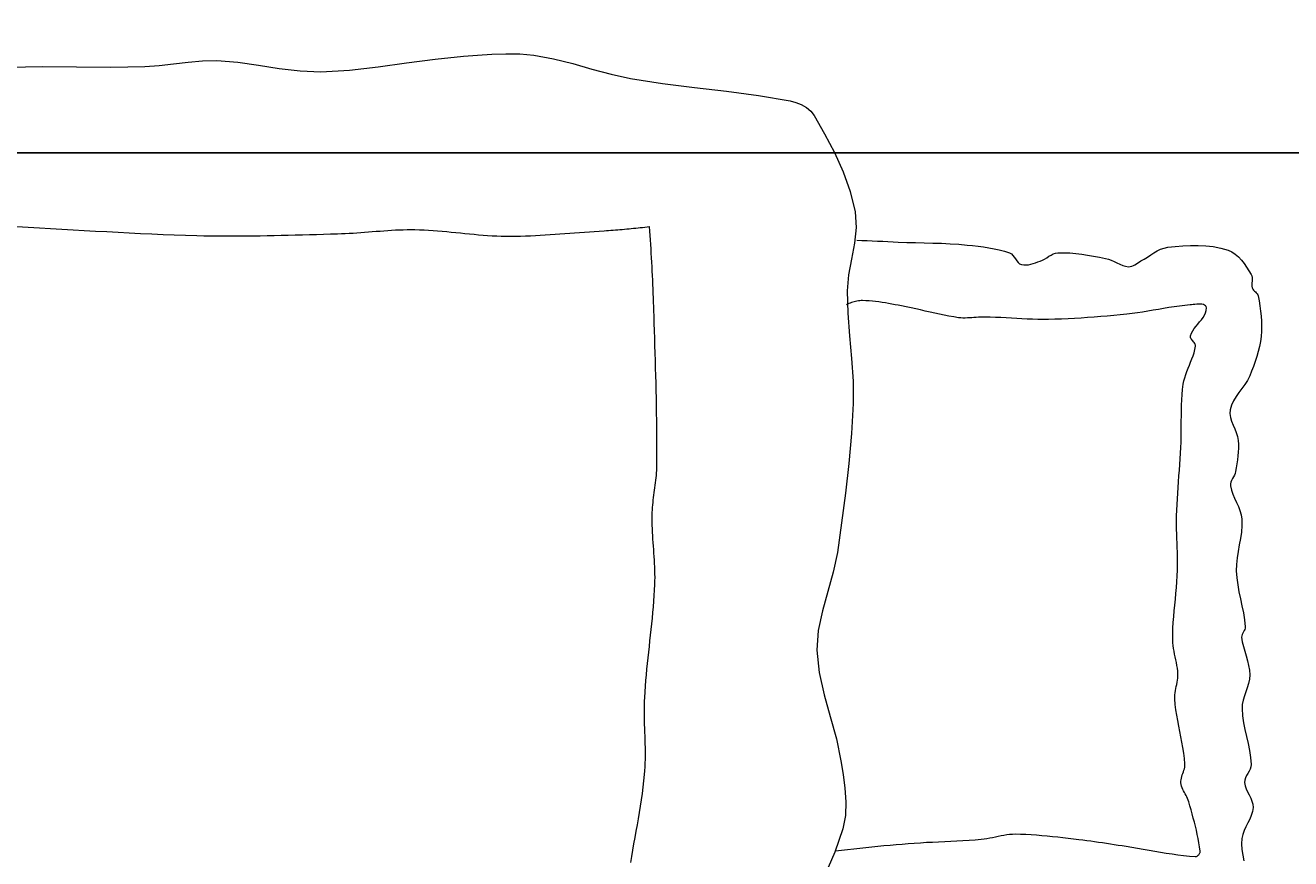
# Model space of a CAD drawing. Units: inches. Extents: x -15 to 423, y -713 to 71.
# Tile 15 of 24: x 308 to 364, y -308 to -270. Entities that reach past the tile are written whole.
import ezdxf

# ---------------------------------------------------------------- set-up
doc = ezdxf.new("R2010")
doc.units = ezdxf.units.IN
doc.header["$MEASUREMENT"] = 0
doc.layers.add('A-ANNO-DIMS', color=2, linetype='Continuous', lineweight=18)
doc.layers.add('A-FURN', color=9, linetype='Continuous', lineweight=13)
doc.styles.get("Standard").update_dxf_attribs({"font": 'arial.ttf'})
doc.dimstyles.get("Standard").update_dxf_attribs({"dimtxt": 0.18, "dimasz": 0.18, "dimexe": 0.18, "dimexo": 0.0625, "dimgap": 0.09, "dimtad": 0, "dimtih": 1, "dimtoh": 1, "dimdec": 0, "dimzin": 0, "dimdsep": 46, "dimlunit": 3, "dimtxsty": 'Standard', "dimcen": 0.09, "dimadec": 0, "dimazin": 0, "dimtfac": 1, "dimtdec": 0, "dimtofl": 0, "dimtmove": 0, "dimatfit": 3, "dimfxl": 1, "dimtolj": 1, "dimtzin": 0, "dimarcsym": 0})

# ---------------------------------------------------------------- blocks, each defined once
blk = doc.blocks.new('BED-DOUBLE')
for p, q in [((51.556, 70.189), (52.201, 70.268)), ((52.201, 70.268), (52.847, 70.326)), ((52.847, 70.326), (53.495, 70.339)), ((53.495, 70.339), (54.428, 70.266)), ((54.428, 70.266), (55.357, 70.134)), ((61.983, 70.229), (63.259, 70.403)), ((63.259, 70.403), (64.539, 70.536)), ((64.539, 70.536), (65.168, 70.585)), ((65.168, 70.585), (65.8, 70.625)), ((65.8, 70.625), (66.431, 70.645)), ((66.431, 70.645), (67.061, 70.633)), ((67.061, 70.633), (67.688, 70.576)), ((67.688, 70.576), (68.563, 70.418)), ((68.563, 70.418), (69.426, 70.201)), ((44.16, 70.042), (45.684, 70.067)), ((45.684, 70.067), (47.211, 70.055)), ((47.211, 70.055), (48.737, 70.043)), ((48.737, 70.043), (50.262, 70.068)), ((50.262, 70.068), (50.909, 70.114)), ((50.909, 70.114), (51.556, 70.189)), ((55.357, 70.134), (56.285, 69.988)), ((56.285, 69.988), (57.214, 69.874)), ((57.214, 69.874), (58.147, 69.837)), ((58.147, 69.837), (59.429, 69.908)), ((59.429, 69.908), (60.707, 70.052)), ((60.707, 70.052), (61.983, 70.229)), ((69.426, 70.201), (70.285, 69.959)), ((70.285, 69.959), (71.146, 69.727)), ((71.146, 69.727), (72.016, 69.538)), ((72.016, 69.538), (73.443, 69.316)), ((73.443, 69.316), (74.876, 69.137)), ((74.876, 69.137), (76.311, 68.967)), ((76.311, 68.967), (77.741, 68.775)), ((77.741, 68.775), (79.163, 68.528)), ((79.163, 68.528), (79.412, 68.464)), ((79.412, 68.464), (79.657, 68.368)), ((79.657, 68.368), (79.885, 68.24)), ((79.885, 68.24), (80.082, 68.078)), ((80.082, 68.078), (80.236, 67.88)), ((80.236, 67.88), (80.703, 67.06)), ((80.703, 67.06), (81.141, 66.219)), ((81.141, 66.219), (81.529, 65.356)), ((81.529, 65.356), (81.847, 64.47)), ((81.847, 64.47), (82.074, 63.56)), ((82.074, 63.56), (82.122, 62.86)), ((44.535, 62.904), (45.039, 62.877)), ((72.754, 62.888), (72.855, 62.9)), ((72.855, 62.9), (72.869, 62.701)), ((45.039, 62.877), (45.543, 62.849)), ((45.543, 62.849), (46.046, 62.82)), ((46.046, 62.82), (46.55, 62.791)), ((46.55, 62.791), (47.053, 62.762)), ((47.053, 62.762), (47.557, 62.732)), ((47.557, 62.732), (48.06, 62.703)), ((48.06, 62.703), (48.564, 62.675)), ((48.564, 62.675), (49.068, 62.647)), ((49.068, 62.647), (49.571, 62.62)), ((49.571, 62.62), (50.075, 62.595)), ((50.075, 62.595), (50.579, 62.572)), ((50.579, 62.572), (51.083, 62.55)), ((51.083, 62.55), (51.586, 62.53)), ((51.586, 62.53), (52.09, 62.513)), ((52.09, 62.513), (52.595, 62.499)), ((52.595, 62.499), (52.909, 62.492)), ((52.909, 62.492), (53.224, 62.487)), ((53.224, 62.487), (53.539, 62.483)), ((53.539, 62.483), (53.854, 62.481)), ((53.854, 62.481), (54.169, 62.481)), ((54.169, 62.481), (54.484, 62.482)), ((54.484, 62.482), (54.799, 62.484)), ((54.799, 62.484), (55.114, 62.488)), ((55.114, 62.488), (55.429, 62.492)), ((55.429, 62.492), (55.744, 62.497)), ((55.744, 62.497), (56.059, 62.504)), ((56.059, 62.504), (56.374, 62.511)), ((56.374, 62.511), (56.689, 62.518)), ((56.689, 62.518), (57.004, 62.526)), ((57.004, 62.526), (57.319, 62.535)), ((57.319, 62.535), (57.634, 62.543)), ((57.634, 62.543), (57.949, 62.552)), ((57.949, 62.552), (58.264, 62.561)), ((58.264, 62.561), (58.579, 62.57)), ((58.579, 62.57), (58.893, 62.579)), ((58.893, 62.579), (59.067, 62.585)), ((59.067, 62.585), (59.24, 62.592)), ((59.24, 62.592), (59.413, 62.602)), ((59.413, 62.602), (59.587, 62.612)), ((59.587, 62.612), (59.76, 62.624)), ((59.76, 62.624), (59.933, 62.637)), ((59.933, 62.637), (60.106, 62.65)), ((60.106, 62.65), (60.279, 62.663)), ((60.279, 62.663), (60.452, 62.677)), ((60.452, 62.677), (60.625, 62.691)), ((60.625, 62.691), (60.798, 62.704)), ((60.798, 62.704), (60.971, 62.717)), ((60.971, 62.717), (61.145, 62.729)), ((61.145, 62.729), (61.318, 62.739)), ((61.318, 62.739), (61.491, 62.749)), ((61.491, 62.749), (61.664, 62.756)), ((61.664, 62.756), (61.837, 62.762)), ((61.837, 62.762), (62.011, 62.766)), ((62.011, 62.766), (62.184, 62.768)), ((62.184, 62.768), (62.357, 62.767)), ((62.357, 62.767), (62.562, 62.762)), ((62.562, 62.762), (62.766, 62.754)), ((62.766, 62.754), (62.969, 62.743)), ((62.969, 62.743), (63.173, 62.73)), ((63.173, 62.73), (63.377, 62.714)), ((63.377, 62.714), (63.58, 62.696)), ((63.58, 62.696), (63.784, 62.677)), ((63.784, 62.677), (63.988, 62.657)), ((63.988, 62.657), (64.191, 62.637)), ((64.191, 62.637), (64.394, 62.616)), ((64.394, 62.616), (64.598, 62.595)), ((64.598, 62.595), (64.801, 62.574)), ((64.801, 62.574), (65.005, 62.555)), ((65.005, 62.555), (65.208, 62.537)), ((65.208, 62.537), (65.412, 62.52)), ((65.412, 62.52), (65.616, 62.505)), ((65.616, 62.505), (65.819, 62.493)), ((65.819, 62.493), (66.023, 62.483)), ((66.023, 62.483), (66.227, 62.476)), ((66.227, 62.476), (66.432, 62.473)), ((66.432, 62.473), (66.652, 62.473)), ((66.652, 62.473), (66.872, 62.475)), ((66.872, 62.475), (67.092, 62.479)), ((67.092, 62.479), (67.312, 62.486)), ((67.312, 62.486), (67.532, 62.494)), ((67.532, 62.494), (67.752, 62.503)), ((67.752, 62.503), (67.972, 62.514)), ((67.972, 62.514), (68.192, 62.527)), ((68.192, 62.527), (68.412, 62.54)), ((68.412, 62.54), (68.632, 62.555)), ((68.632, 62.555), (68.852, 62.57)), ((68.852, 62.57), (69.072, 62.586)), ((69.072, 62.586), (69.291, 62.602)), ((69.291, 62.602), (69.511, 62.619)), ((69.511, 62.619), (69.731, 62.636)), ((69.731, 62.636), (69.951, 62.652)), ((69.951, 62.652), (70.17, 62.669)), ((70.17, 62.669), (70.39, 62.685)), ((70.39, 62.685), (70.61, 62.701)), ((70.61, 62.701), (70.83, 62.716)), ((70.83, 62.716), (70.931, 62.723)), ((70.931, 62.723), (71.033, 62.73)), ((71.033, 62.73), (71.134, 62.737)), ((71.134, 62.737), (71.236, 62.745)), ((71.236, 62.745), (71.337, 62.753)), ((71.337, 62.753), (71.438, 62.761)), ((71.438, 62.761), (71.54, 62.769)), ((71.54, 62.769), (71.641, 62.778)), ((71.641, 62.778), (71.742, 62.787)), ((71.742, 62.787), (71.844, 62.796)), ((71.844, 62.796), (71.945, 62.805)), ((71.945, 62.805), (72.046, 62.814)), ((72.046, 62.814), (72.147, 62.824)), ((72.147, 62.824), (72.249, 62.834)), ((72.249, 62.834), (72.35, 62.845)), ((72.35, 62.845), (72.451, 62.855)), ((72.451, 62.855), (72.552, 62.866)), ((72.552, 62.866), (72.653, 62.877)), ((72.653, 62.877), (72.754, 62.888)), ((72.869, 62.701), (72.882, 62.501)), ((72.882, 62.501), (72.894, 62.302)), ((82.122, 62.86), (82.046, 62.156)), ((72.894, 62.302), (72.906, 62.103)), ((72.906, 62.103), (72.918, 61.903)), ((72.918, 61.903), (72.929, 61.704)), ((82.046, 62.156), (81.91, 61.449)), ((82.14, 62.295), (82.373, 62.284)), ((82.373, 62.284), (82.606, 62.273)), ((82.606, 62.273), (82.839, 62.263)), ((82.839, 62.263), (83.072, 62.252)), ((83.072, 62.252), (83.305, 62.242)), ((83.305, 62.242), (83.538, 62.231)), ((83.538, 62.231), (83.771, 62.221)), ((83.771, 62.221), (84.004, 62.21)), ((84.004, 62.21), (84.39, 62.196)), ((84.39, 62.196), (84.776, 62.185)), ((84.776, 62.185), (85.163, 62.175)), ((85.163, 62.175), (85.549, 62.165)), ((85.549, 62.165), (85.935, 62.152)), ((85.935, 62.152), (86.321, 62.134)), ((86.321, 62.134), (86.706, 62.11)), ((86.706, 62.11), (87.091, 62.077)), ((87.091, 62.077), (87.331, 62.053)), ((87.331, 62.053), (87.572, 62.025)), ((87.572, 62.025), (87.812, 61.994)), ((87.812, 61.994), (88.052, 61.957)), ((88.052, 61.957), (88.29, 61.912)), ((88.29, 61.912), (88.525, 61.859)), ((88.525, 61.859), (88.758, 61.795)), ((88.758, 61.795), (88.987, 61.72)), ((95.451, 61.723), (95.598, 61.81)), ((95.598, 61.81), (95.748, 61.884)), ((95.748, 61.884), (95.904, 61.941)), ((95.904, 61.941), (96.067, 61.975)), ((96.067, 61.975), (96.405, 62.013)), ((96.405, 62.013), (96.745, 62.042)), ((96.745, 62.042), (97.088, 62.058)), ((97.088, 62.058), (97.43, 62.06)), ((97.43, 62.06), (97.771, 62.042)), ((97.771, 62.042), (98.108, 62.004)), ((98.108, 62.004), (98.441, 61.941)), ((98.441, 61.941), (98.766, 61.851)), ((98.766, 61.851), (98.937, 61.777)), ((98.937, 61.777), (99.092, 61.674)), ((72.929, 61.704), (72.94, 61.505)), ((72.94, 61.505), (72.951, 61.305)), ((72.951, 61.305), (72.961, 61.106)), ((81.91, 61.449), (81.779, 60.741)), ((88.987, 61.72), (89.067, 61.676)), ((89.067, 61.676), (89.134, 61.612)), ((89.134, 61.612), (89.194, 61.536)), ((89.194, 61.536), (89.25, 61.453)), ((89.25, 61.453), (89.306, 61.371)), ((89.306, 61.371), (89.367, 61.298)), ((89.367, 61.298), (89.436, 61.239)), ((89.436, 61.239), (89.518, 61.202)), ((89.518, 61.202), (89.622, 61.184)), ((89.727, 61.183), (89.833, 61.195)), ((89.833, 61.195), (89.94, 61.219)), ((89.94, 61.219), (90.046, 61.25)), ((90.046, 61.25), (90.151, 61.285)), ((90.151, 61.285), (90.255, 61.321)), ((90.255, 61.321), (90.358, 61.356)), ((90.358, 61.356), (90.459, 61.397)), ((90.459, 61.397), (90.556, 61.45)), ((90.556, 61.45), (90.651, 61.509)), ((90.651, 61.509), (90.746, 61.57)), ((90.746, 61.57), (90.841, 61.627)), ((90.841, 61.627), (90.938, 61.675)), ((90.938, 61.675), (91.039, 61.71)), ((91.039, 61.71), (91.144, 61.726)), ((91.144, 61.726), (91.412, 61.729)), ((91.412, 61.729), (91.68, 61.719)), ((91.68, 61.719), (91.948, 61.697)), ((91.948, 61.697), (92.215, 61.665)), ((92.215, 61.665), (92.481, 61.626)), ((92.481, 61.626), (92.747, 61.58)), ((92.747, 61.58), (93.012, 61.531)), ((93.012, 61.531), (93.276, 61.479)), ((93.276, 61.479), (93.409, 61.444)), ((93.409, 61.444), (93.539, 61.395)), ((93.539, 61.395), (93.667, 61.337)), ((93.667, 61.337), (93.794, 61.275)), ((93.794, 61.275), (93.921, 61.216)), ((93.921, 61.216), (94.05, 61.164)), ((94.531, 61.156), (94.599, 61.194)), ((94.599, 61.194), (94.666, 61.238)), ((94.666, 61.238), (94.733, 61.282)), ((94.733, 61.282), (94.799, 61.325)), ((94.799, 61.325), (94.867, 61.363)), ((94.867, 61.363), (95.016, 61.444)), ((95.016, 61.444), (95.161, 61.535)), ((95.161, 61.535), (95.306, 61.63)), ((95.306, 61.63), (95.451, 61.723)), ((99.092, 61.674), (99.234, 61.548)), ((99.234, 61.548), (99.365, 61.405)), ((99.365, 61.405), (99.485, 61.248)), ((99.485, 61.248), (99.598, 61.085)), ((72.961, 61.106), (72.971, 60.906)), ((72.971, 60.906), (72.981, 60.707)), ((72.981, 60.707), (72.99, 60.507)), ((81.779, 60.741), (81.716, 60.031)), ((89.622, 61.184), (89.727, 61.183)), ((94.05, 61.164), (94.181, 61.125)), ((94.181, 61.125), (94.316, 61.104)), ((94.316, 61.104), (94.391, 61.107)), ((94.391, 61.107), (94.462, 61.126)), ((94.462, 61.126), (94.531, 61.156)), ((99.598, 61.085), (99.705, 60.919)), ((99.705, 60.919), (99.808, 60.757)), ((99.808, 60.757), (99.838, 60.69)), ((99.838, 60.69), (99.852, 60.618)), ((72.99, 60.507), (72.999, 60.308)), ((72.999, 60.308), (73.007, 60.108)), ((73.007, 60.108), (73.015, 59.909)), ((99.839, 60.384), (99.834, 60.305)), ((99.834, 60.305), (99.836, 60.227)), ((99.836, 60.227), (99.852, 60.153)), ((99.847, 60.463), (99.839, 60.384)), ((99.853, 60.542), (99.847, 60.463)), ((99.852, 60.618), (99.853, 60.542)), ((99.852, 60.153), (99.875, 60.104)), ((99.875, 60.104), (99.908, 60.059)), ((99.908, 60.059), (99.948, 60.017)), ((73.015, 59.909), (73.023, 59.709)), ((73.023, 59.709), (73.03, 59.51)), ((73.03, 59.51), (73.037, 59.31)), ((81.716, 60.031), (81.743, 59.019)), ((81.908, 59.5), (81.849, 59.477)), ((81.968, 59.521), (81.908, 59.5)), ((82.029, 59.539), (81.968, 59.521)), ((82.091, 59.554), (82.029, 59.539)), ((82.153, 59.567), (82.091, 59.554)), ((82.216, 59.576), (82.153, 59.567)), ((82.279, 59.583), (82.216, 59.576)), ((82.342, 59.586), (82.279, 59.583)), ((82.405, 59.587), (82.342, 59.586)), ((82.551, 59.582), (82.405, 59.587)), ((82.697, 59.573), (82.551, 59.582)), ((82.843, 59.56), (82.697, 59.573)), ((82.989, 59.544), (82.843, 59.56)), ((83.134, 59.525), (82.989, 59.544)), ((83.28, 59.503), (83.134, 59.525)), ((83.425, 59.48), (83.28, 59.503)), ((99.948, 60.017), (99.99, 59.977)), ((99.99, 59.977), (100.032, 59.936)), ((100.032, 59.936), (100.069, 59.894)), ((100.069, 59.894), (100.098, 59.848)), ((100.098, 59.848), (100.115, 59.797)), ((100.115, 59.797), (100.154, 59.573)), ((100.154, 59.573), (100.19, 59.348)), ((73.037, 59.31), (73.044, 59.111)), ((73.044, 59.111), (73.05, 58.911)), ((81.735, 59.422), (81.681, 59.391)), ((81.791, 59.451), (81.735, 59.422)), ((81.743, 59.019), (81.82, 58.007)), ((81.849, 59.477), (81.791, 59.451)), ((83.57, 59.455), (83.425, 59.48)), ((83.715, 59.429), (83.57, 59.455)), ((83.859, 59.403), (83.715, 59.429)), ((84.004, 59.376), (83.859, 59.403)), ((84.148, 59.35), (84.004, 59.376)), ((84.362, 59.31), (84.148, 59.35)), ((84.574, 59.266), (84.362, 59.31)), ((84.787, 59.219), (84.574, 59.266)), ((84.999, 59.171), (84.787, 59.219)), ((85.21, 59.121), (84.999, 59.171)), ((85.422, 59.072), (85.21, 59.121)), ((85.634, 59.023), (85.422, 59.072)), ((85.846, 58.976), (85.634, 59.023)), ((86.059, 58.931), (85.846, 58.976)), ((86.272, 58.89), (86.059, 58.931)), ((93.943, 58.949), (93.651, 58.921)), ((94.235, 58.978), (93.943, 58.949)), ((94.472, 59.005), (94.235, 58.978)), ((94.708, 59.038), (94.472, 59.005)), ((94.944, 59.074), (94.708, 59.038)), ((95.179, 59.113), (94.944, 59.074)), ((95.414, 59.154), (95.179, 59.113)), ((95.649, 59.195), (95.414, 59.154)), ((95.884, 59.236), (95.649, 59.195)), ((96.119, 59.275), (95.884, 59.236)), ((96.354, 59.312), (96.119, 59.275)), ((96.59, 59.345), (96.354, 59.312)), ((96.826, 59.373), (96.59, 59.345)), ((97.064, 59.395), (96.826, 59.373)), ((97.13, 59.401), (97.064, 59.395)), ((97.204, 59.409), (97.13, 59.401)), ((97.283, 59.417), (97.204, 59.409)), ((97.364, 59.424), (97.283, 59.417)), ((97.444, 59.429), (97.364, 59.424)), ((97.523, 59.429), (97.444, 59.429)), ((97.596, 59.423), (97.523, 59.429)), ((97.661, 59.411), (97.596, 59.423)), ((97.648, 58.827), (97.71, 58.929)), ((97.717, 59.389), (97.661, 59.411)), ((97.71, 58.929), (97.758, 59.034)), ((97.76, 59.358), (97.717, 59.389)), ((97.758, 59.034), (97.789, 59.144)), ((97.788, 59.316), (97.76, 59.358)), ((97.799, 59.261), (97.788, 59.316)), ((97.789, 59.144), (97.799, 59.261)), ((100.19, 59.348), (100.221, 59.121)), ((100.221, 59.121), (100.245, 58.894)), ((73.05, 58.911), (73.06, 58.576)), ((73.06, 58.576), (73.07, 58.24)), ((86.486, 58.853), (86.272, 58.89)), ((86.701, 58.821), (86.486, 58.853)), ((86.799, 58.811), (86.701, 58.821)), ((86.897, 58.806), (86.799, 58.811)), ((86.996, 58.805), (86.897, 58.806)), ((87.095, 58.808), (86.996, 58.805)), ((87.193, 58.813), (87.095, 58.808)), ((87.292, 58.819), (87.193, 58.813)), ((87.392, 58.827), (87.292, 58.819)), ((87.491, 58.835), (87.392, 58.827)), ((87.59, 58.842), (87.491, 58.835)), ((87.689, 58.848), (87.59, 58.842)), ((87.788, 58.851), (87.689, 58.848)), ((87.887, 58.851), (87.788, 58.851)), ((88.123, 58.845), (87.887, 58.851)), ((88.359, 58.835), (88.123, 58.845)), ((88.596, 58.824), (88.359, 58.835)), ((88.832, 58.81), (88.596, 58.824)), ((89.068, 58.797), (88.832, 58.81)), ((89.304, 58.783), (89.068, 58.797)), ((89.54, 58.77), (89.304, 58.783)), ((89.777, 58.758), (89.54, 58.77)), ((90.013, 58.749), (89.777, 58.758)), ((90.249, 58.743), (90.013, 58.749)), ((90.485, 58.741), (90.249, 58.743)), ((90.722, 58.743), (90.485, 58.741)), ((91.015, 58.75), (90.722, 58.743)), ((91.308, 58.76), (91.015, 58.75)), ((91.602, 58.773), (91.308, 58.76)), ((91.895, 58.788), (91.602, 58.773)), ((92.188, 58.805), (91.895, 58.788)), ((92.481, 58.824), (92.188, 58.805)), ((92.774, 58.846), (92.481, 58.824)), ((93.066, 58.869), (92.774, 58.846)), ((93.359, 58.894), (93.066, 58.869)), ((93.651, 58.921), (93.359, 58.894)), ((97.256, 58.336), (97.333, 58.436)), ((97.333, 58.436), (97.414, 58.534)), ((97.414, 58.534), (97.496, 58.631)), ((97.496, 58.631), (97.575, 58.728)), ((97.575, 58.728), (97.648, 58.827)), ((100.245, 58.894), (100.261, 58.667)), ((100.261, 58.667), (100.267, 58.439)), ((100.267, 58.439), (100.263, 58.213)), ((73.07, 58.24), (73.081, 57.905)), ((73.081, 57.905), (73.091, 57.57)), ((81.82, 58.007), (81.91, 56.995)), ((97.083, 57.974), (97.088, 58.015)), ((97.09, 57.934), (97.083, 57.974)), ((97.088, 58.015), (97.13, 58.127)), ((97.106, 57.895), (97.09, 57.934)), ((97.13, 57.856), (97.106, 57.895)), ((97.13, 58.127), (97.187, 58.233)), ((97.159, 57.818), (97.13, 57.856)), ((97.191, 57.78), (97.159, 57.818)), ((97.187, 58.233), (97.256, 58.336)), ((100.246, 57.986), (100.215, 57.758)), ((100.263, 58.213), (100.246, 57.986)), ((73.091, 57.57), (73.101, 57.234)), ((73.101, 57.234), (73.111, 56.899)), ((97.223, 57.743), (97.191, 57.78)), ((97.199, 57.112), (97.245, 57.254)), ((97.253, 57.704), (97.223, 57.743)), ((97.245, 57.254), (97.282, 57.397)), ((97.28, 57.666), (97.253, 57.704)), ((97.299, 57.626), (97.28, 57.666)), ((97.282, 57.397), (97.31, 57.543)), ((97.31, 57.585), (97.299, 57.626)), ((97.31, 57.543), (97.31, 57.585)), ((100.119, 57.305), (100.056, 57.082)), ((100.172, 57.53), (100.119, 57.305)), ((100.215, 57.758), (100.172, 57.53)), ((73.111, 56.899), (73.121, 56.563)), ((81.91, 56.995), (81.976, 55.984)), ((96.978, 56.556), (97.036, 56.695)), ((97.036, 56.695), (97.093, 56.833)), ((97.093, 56.833), (97.148, 56.972)), ((97.148, 56.972), (97.199, 57.112)), ((99.985, 56.861), (99.907, 56.642)), ((100.056, 57.082), (99.985, 56.861)), ((73.121, 56.563), (73.13, 56.228)), ((73.13, 56.228), (73.139, 55.893)), ((96.79, 55.992), (96.827, 56.135)), ((96.827, 56.135), (96.872, 56.276)), ((96.872, 56.276), (96.923, 56.417)), ((96.923, 56.417), (96.978, 56.556)), ((99.736, 56.211), (99.638, 56.015)), ((99.824, 56.425), (99.736, 56.211)), ((99.907, 56.642), (99.824, 56.425)), ((73.139, 55.893), (73.147, 55.557)), ((73.147, 55.557), (73.154, 55.222)), ((81.976, 55.984), (81.981, 54.972)), ((96.712, 55.377), (96.734, 55.611)), ((96.734, 55.611), (96.763, 55.846)), ((96.763, 55.846), (96.79, 55.992)), ((99.388, 55.647), (99.254, 55.467)), ((99.519, 55.828), (99.388, 55.647)), ((99.638, 56.015), (99.519, 55.828)), ((73.154, 55.222), (73.161, 54.886)), ((81.981, 54.972), (81.907, 53.633)), ((96.686, 54.905), (96.696, 55.141)), ((96.696, 55.141), (96.712, 55.377)), ((99.012, 55.1), (98.921, 54.904)), ((99.125, 55.286), (99.012, 55.1)), ((99.254, 55.467), (99.125, 55.286)), ((73.161, 54.886), (73.167, 54.551)), ((73.167, 54.551), (73.172, 54.215)), ((96.675, 54.195), (96.677, 54.432)), ((96.677, 54.432), (96.68, 54.668)), ((96.68, 54.668), (96.686, 54.905)), ((98.864, 54.697), (98.853, 54.524)), ((98.853, 54.524), (98.878, 54.353)), ((98.921, 54.904), (98.864, 54.697)), ((73.172, 54.215), (73.176, 53.88)), ((73.176, 53.88), (73.179, 53.545)), ((96.674, 53.721), (96.675, 53.958)), ((96.675, 53.958), (96.675, 54.195)), ((98.878, 54.353), (98.928, 54.183)), ((98.928, 54.183), (98.994, 54.014)), ((98.994, 54.014), (99.066, 53.845)), ((99.066, 53.845), (99.134, 53.674)), ((73.179, 53.545), (73.181, 53.209)), ((81.907, 53.633), (81.79, 52.296)), ((96.665, 53.247), (96.671, 53.484)), ((96.671, 53.484), (96.674, 53.721)), ((99.134, 53.674), (99.188, 53.502)), ((99.188, 53.502), (99.219, 53.328)), ((99.219, 53.328), (99.229, 53.153)), ((73.181, 52.874), (73.18, 52.538)), ((73.181, 53.209), (73.181, 52.874)), ((96.625, 52.5), (96.641, 52.755)), ((96.641, 52.755), (96.656, 53.011)), ((96.656, 53.011), (96.665, 53.247)), ((99.222, 52.803), (99.207, 52.628)), ((99.23, 52.978), (99.222, 52.803)), ((99.229, 53.153), (99.23, 52.978)), ((73.178, 52.203), (73.176, 52.092)), ((73.18, 52.538), (73.178, 52.203)), ((81.79, 52.296), (81.64, 50.963)), ((96.589, 51.989), (96.608, 52.244)), ((96.608, 52.244), (96.625, 52.5)), ((99.163, 52.278), (99.136, 52.104)), ((99.187, 52.453), (99.163, 52.278)), ((99.207, 52.628), (99.187, 52.453)), ((73.144, 51.649), (73.132, 51.539)), ((73.155, 51.76), (73.144, 51.649)), ((73.164, 51.87), (73.155, 51.76)), ((73.171, 51.981), (73.164, 51.87)), ((73.176, 52.092), (73.171, 51.981)), ((96.551, 51.478), (96.57, 51.734)), ((96.57, 51.734), (96.589, 51.989)), ((98.968, 51.614), (98.928, 51.536)), ((99.01, 51.691), (98.968, 51.614)), ((99.051, 51.769), (99.01, 51.691)), ((99.085, 51.849), (99.051, 51.769)), ((99.107, 51.931), (99.085, 51.849)), ((99.136, 52.104), (99.107, 51.931)), ((73.076, 51.098), (73.061, 50.987)), ((73.09, 51.208), (73.076, 51.098)), ((73.105, 51.318), (73.09, 51.208)), ((73.119, 51.428), (73.105, 51.318)), ((73.132, 51.539), (73.119, 51.428)), ((96.515, 50.968), (96.533, 51.223)), ((96.533, 51.223), (96.551, 51.478)), ((98.896, 51.458), (98.878, 51.378)), ((98.878, 51.378), (98.878, 51.295)), ((98.878, 51.295), (98.918, 51.103)), ((98.928, 51.536), (98.896, 51.458)), ((98.918, 51.103), (98.981, 50.917)), ((72.995, 50.435), (72.985, 50.325)), ((73.006, 50.546), (72.995, 50.435)), ((73.018, 50.656), (73.006, 50.546)), ((73.032, 50.767), (73.018, 50.656)), ((73.046, 50.877), (73.032, 50.767)), ((73.061, 50.987), (73.046, 50.877)), ((81.64, 50.963), (81.466, 49.632)), ((96.473, 50.201), (96.485, 50.456)), ((96.485, 50.456), (96.499, 50.712)), ((96.499, 50.712), (96.515, 50.968)), ((98.981, 50.917), (99.059, 50.733)), ((99.059, 50.733), (99.144, 50.552)), ((99.144, 50.552), (99.228, 50.37)), ((72.969, 49.992), (72.967, 49.837)), ((72.972, 50.103), (72.969, 49.992)), ((72.977, 50.214), (72.972, 50.103)), ((72.985, 50.325), (72.977, 50.214)), ((96.461, 49.743), (96.464, 49.945)), ((96.464, 49.945), (96.473, 50.201)), ((99.228, 50.37), (99.301, 50.186)), ((99.301, 50.186), (99.357, 49.999)), ((99.357, 49.999), (99.386, 49.806)), ((72.967, 49.837), (72.969, 49.681)), ((72.969, 49.681), (72.973, 49.525)), ((72.973, 49.525), (72.978, 49.37)), ((72.978, 49.37), (72.986, 49.214)), ((81.466, 49.632), (81.275, 48.303)), ((96.461, 49.54), (96.461, 49.743)), ((96.464, 49.337), (96.461, 49.54)), ((96.47, 49.135), (96.464, 49.337)), ((99.389, 49.514), (99.365, 49.224)), ((99.386, 49.806), (99.389, 49.514)), ((72.986, 49.214), (72.995, 49.058)), ((72.995, 49.058), (73.004, 48.903)), ((73.004, 48.903), (73.015, 48.747)), ((73.015, 48.747), (73.026, 48.591)), ((96.477, 48.932), (96.47, 49.135)), ((96.484, 48.73), (96.477, 48.932)), ((96.492, 48.527), (96.484, 48.73)), ((99.323, 48.933), (99.271, 48.643)), ((99.365, 49.224), (99.323, 48.933)), ((73.026, 48.591), (73.037, 48.436)), ((73.037, 48.436), (73.048, 48.28)), ((73.048, 48.28), (73.059, 48.125)), ((81.275, 48.303), (81.093, 47.426)), ((96.499, 48.325), (96.492, 48.527)), ((96.504, 48.122), (96.499, 48.325)), ((99.217, 48.353), (99.171, 48.063)), ((99.271, 48.643), (99.217, 48.353)), ((73.059, 48.125), (73.068, 47.969)), ((73.068, 47.969), (73.077, 47.813)), ((73.077, 47.813), (73.084, 47.658)), ((73.084, 47.658), (73.09, 47.502)), ((96.502, 47.515), (96.506, 47.717)), ((96.507, 47.92), (96.504, 48.122)), ((96.506, 47.717), (96.507, 47.92)), ((99.141, 47.772), (99.135, 47.48)), ((99.171, 48.063), (99.141, 47.772)), ((73.092, 47.035), (73.087, 46.88)), ((73.09, 47.502), (73.093, 47.347)), ((73.094, 47.191), (73.092, 47.035)), ((73.093, 47.347), (73.094, 47.191)), ((81.093, 47.426), (80.849, 46.558)), ((96.475, 46.994), (96.491, 47.254)), ((96.491, 47.254), (96.502, 47.515)), ((99.135, 47.48), (99.157, 47.165)), ((99.157, 47.165), (99.2, 46.852)), ((73.075, 46.626), (73.06, 46.373)), ((73.087, 46.88), (73.075, 46.626)), ((80.849, 46.558), (80.603, 45.691)), ((96.407, 46.213), (96.432, 46.473)), ((96.432, 46.473), (96.455, 46.733)), ((96.455, 46.733), (96.475, 46.994)), ((99.2, 46.852), (99.257, 46.541)), ((99.257, 46.541), (99.322, 46.23)), ((73.042, 46.119), (73.022, 45.866)), ((73.06, 46.373), (73.042, 46.119)), ((96.358, 45.693), (96.382, 45.953)), ((96.382, 45.953), (96.407, 46.213)), ((99.322, 46.23), (99.389, 45.92)), ((99.389, 45.92), (99.452, 45.609)), ((72.976, 45.36), (72.95, 45.107)), ((73, 45.613), (72.976, 45.36)), ((73.022, 45.866), (73, 45.613)), ((80.603, 45.691), (80.417, 44.818)), ((96.317, 45.173), (96.336, 45.433)), ((96.336, 45.433), (96.358, 45.693)), ((99.452, 45.609), (99.505, 45.296)), ((72.924, 44.854), (72.897, 44.601)), ((72.95, 45.107), (72.924, 44.854)), ((80.417, 44.818), (80.352, 43.933)), ((96.293, 44.652), (96.302, 44.912)), ((96.302, 44.912), (96.317, 45.173)), ((99.489, 44.807), (99.456, 44.751)), ((99.518, 44.864), (99.489, 44.807)), ((99.505, 45.296), (99.54, 44.982)), ((99.536, 44.922), (99.518, 44.864)), ((99.54, 44.982), (99.536, 44.922)), ((72.869, 44.349), (72.841, 44.096)), ((72.897, 44.601), (72.869, 44.349)), ((96.29, 44.391), (96.293, 44.652)), ((96.295, 44.263), (96.29, 44.391)), ((96.307, 44.136), (96.295, 44.263)), ((99.377, 44.58), (99.374, 44.52)), ((99.374, 44.52), (99.405, 44.305)), ((99.395, 44.638), (99.377, 44.58)), ((99.423, 44.695), (99.395, 44.638)), ((99.405, 44.305), (99.453, 44.092)), ((99.456, 44.751), (99.423, 44.695)), ((72.813, 43.843), (72.785, 43.591)), ((72.841, 44.096), (72.813, 43.843)), ((80.352, 43.933), (80.453, 42.928)), ((96.325, 44.009), (96.307, 44.136)), ((96.348, 43.882), (96.325, 44.009)), ((96.374, 43.756), (96.348, 43.882)), ((96.402, 43.63), (96.374, 43.756)), ((96.43, 43.504), (96.402, 43.63)), ((99.453, 44.092), (99.512, 43.881)), ((99.512, 43.881), (99.576, 43.671)), ((99.576, 43.671), (99.637, 43.46)), ((72.733, 43.085), (72.709, 42.832)), ((72.759, 43.338), (72.733, 43.085)), ((72.785, 43.591), (72.759, 43.338)), ((96.457, 43.378), (96.43, 43.504)), ((96.481, 43.251), (96.457, 43.378)), ((96.502, 43.124), (96.481, 43.251)), ((96.517, 42.997), (96.502, 43.124)), ((99.637, 43.46), (99.689, 43.249)), ((99.689, 43.249), (99.726, 43.036)), ((72.687, 42.579), (72.667, 42.325)), ((72.709, 42.832), (72.687, 42.579)), ((80.453, 42.928), (80.676, 41.938)), ((96.468, 42.4), (96.487, 42.494)), ((96.487, 42.494), (96.504, 42.587)), ((96.504, 42.587), (96.517, 42.681)), ((96.525, 42.869), (96.517, 42.997)), ((96.517, 42.681), (96.525, 42.775)), ((96.525, 42.775), (96.525, 42.869)), ((99.726, 42.628), (99.686, 42.439)), ((99.726, 43.036), (99.74, 42.82)), ((99.74, 42.82), (99.726, 42.628)), ((72.649, 42.072), (72.634, 41.818)), ((72.667, 42.325), (72.649, 42.072)), ((80.676, 41.938), (80.958, 40.954)), ((96.378, 41.839), (96.383, 41.933)), ((96.383, 41.933), (96.393, 42.027)), ((96.393, 42.027), (96.409, 42.12)), ((96.409, 42.12), (96.427, 42.214)), ((96.427, 42.214), (96.447, 42.307)), ((96.447, 42.307), (96.468, 42.4)), ((99.565, 42.066), (99.5, 41.88)), ((99.63, 42.252), (99.565, 42.066)), ((99.686, 42.439), (99.63, 42.252)), ((72.621, 41.473), (72.619, 41.3)), ((72.626, 41.646), (72.621, 41.473)), ((72.634, 41.818), (72.626, 41.646)), ((96.381, 41.746), (96.378, 41.839)), ((96.405, 41.502), (96.381, 41.746)), ((96.436, 41.259), (96.405, 41.502)), ((99.406, 41.504), (99.393, 41.313)), ((99.444, 41.693), (99.406, 41.504)), ((99.5, 41.88), (99.444, 41.693)), ((72.619, 41.3), (72.62, 41.127)), ((72.62, 41.127), (72.622, 40.954)), ((72.622, 40.954), (72.625, 40.78)), ((80.958, 40.954), (81.233, 39.968)), ((96.474, 41.016), (96.436, 41.259)), ((96.516, 40.775), (96.474, 41.016)), ((99.393, 41.313), (99.412, 40.998)), ((99.412, 40.998), (99.457, 40.685)), ((72.625, 40.78), (72.63, 40.607)), ((72.63, 40.607), (72.636, 40.434)), ((72.636, 40.434), (72.642, 40.261)), ((72.642, 40.261), (72.648, 40.088)), ((96.562, 40.533), (96.516, 40.775)), ((96.609, 40.292), (96.562, 40.533)), ((96.656, 40.051), (96.609, 40.292)), ((99.457, 40.685), (99.519, 40.374)), ((99.519, 40.374), (99.589, 40.064)), ((72.648, 40.088), (72.654, 39.914)), ((72.654, 39.914), (72.659, 39.741)), ((72.659, 39.741), (72.662, 39.568)), ((81.233, 39.968), (81.436, 38.971)), ((96.702, 39.81), (96.656, 40.051)), ((96.744, 39.568), (96.702, 39.81)), ((99.589, 40.064), (99.661, 39.753)), ((99.661, 39.753), (99.724, 39.442)), ((72.662, 39.568), (72.665, 39.395)), ((72.665, 39.222), (72.664, 39.049)), ((72.665, 39.395), (72.665, 39.222)), ((96.782, 39.326), (96.744, 39.568)), ((96.812, 39.083), (96.782, 39.326)), ((99.724, 39.442), (99.773, 39.13)), ((99.773, 39.13), (99.798, 38.815)), ((72.641, 38.531), (72.627, 38.359)), ((72.652, 38.704), (72.641, 38.531)), ((72.659, 38.877), (72.652, 38.704)), ((72.664, 39.049), (72.659, 38.877)), ((81.436, 38.971), (81.528, 38.364)), ((96.769, 38.483), (96.792, 38.554)), ((96.792, 38.554), (96.812, 38.624)), ((96.835, 38.839), (96.812, 39.083)), ((96.812, 38.624), (96.827, 38.695)), ((96.827, 38.695), (96.836, 38.767)), ((96.836, 38.767), (96.835, 38.839)), ((99.755, 38.608), (99.707, 38.509)), ((99.788, 38.71), (99.755, 38.608)), ((99.798, 38.815), (99.788, 38.71)), ((72.598, 38.076), (72.565, 37.793)), ((72.627, 38.359), (72.598, 38.076)), ((81.528, 38.364), (81.611, 37.75)), ((96.657, 38.06), (96.663, 38.131)), ((96.659, 37.988), (96.657, 38.06)), ((96.671, 37.913), (96.659, 37.988)), ((96.663, 38.131), (96.677, 38.202)), ((96.677, 38.202), (96.696, 38.272)), ((96.696, 38.272), (96.719, 38.343)), ((96.719, 38.343), (96.744, 38.413)), ((96.744, 38.413), (96.769, 38.483)), ((99.516, 38.111), (99.507, 38.006)), ((99.507, 38.006), (99.529, 37.861)), ((99.548, 38.213), (99.516, 38.111)), ((99.596, 38.312), (99.548, 38.213)), ((99.651, 38.41), (99.596, 38.312)), ((99.707, 38.509), (99.651, 38.41)), ((72.528, 37.51), (72.488, 37.228)), ((72.565, 37.793), (72.528, 37.51)), ((81.611, 37.75), (81.655, 37.136)), ((96.69, 37.84), (96.671, 37.913)), ((96.715, 37.769), (96.69, 37.84)), ((96.745, 37.699), (96.715, 37.769)), ((96.778, 37.63), (96.745, 37.699)), ((96.814, 37.562), (96.778, 37.63)), ((96.851, 37.494), (96.814, 37.562)), ((96.887, 37.425), (96.851, 37.494)), ((96.923, 37.357), (96.887, 37.425)), ((99.529, 37.861), (99.576, 37.721)), ((99.576, 37.721), (99.64, 37.583)), ((99.64, 37.583), (99.711, 37.447)), ((99.711, 37.447), (99.78, 37.311)), ((72.445, 36.947), (72.399, 36.665)), ((72.488, 37.228), (72.445, 36.947)), ((81.655, 37.136), (81.634, 36.529)), ((96.955, 37.287), (96.923, 37.357)), ((96.984, 37.216), (96.955, 37.287)), ((97.008, 37.144), (96.984, 37.216)), ((97.059, 36.962), (97.008, 37.144)), ((97.11, 36.78), (97.059, 36.962)), ((99.78, 37.311), (99.838, 37.174)), ((99.838, 37.174), (99.877, 37.034)), ((99.888, 36.889), (99.862, 36.708)), ((99.877, 37.034), (99.888, 36.889)), ((72.352, 36.384), (72.303, 36.103)), ((72.399, 36.665), (72.352, 36.384)), ((81.634, 36.529), (81.518, 35.937)), ((97.161, 36.597), (97.11, 36.78)), ((97.211, 36.414), (97.161, 36.597)), ((97.26, 36.231), (97.211, 36.414)), ((99.737, 36.363), (99.654, 36.194)), ((99.809, 36.534), (99.737, 36.363)), ((99.862, 36.708), (99.809, 36.534)), ((72.254, 35.822), (72.204, 35.541)), ((72.303, 36.103), (72.254, 35.822)), ((81.518, 35.937), (81.158, 34.884)), ((88.982, 35.686), (89.109, 35.697)), ((89.109, 35.697), (89.237, 35.7)), ((89.237, 35.7), (89.476, 35.697)), ((89.476, 35.697), (89.714, 35.689)), ((97.306, 36.048), (97.26, 36.231)), ((97.35, 35.864), (97.306, 36.048)), ((97.391, 35.68), (97.35, 35.864)), ((99.49, 35.855), (99.427, 35.681)), ((99.569, 36.025), (99.49, 35.855)), ((99.654, 36.194), (99.569, 36.025)), ((72.153, 35.261), (72.103, 34.98)), ((72.204, 35.541), (72.153, 35.261)), ((82.818, 35.125), (83.089, 35.152)), ((83.089, 35.152), (83.36, 35.178)), ((83.36, 35.178), (83.631, 35.203)), ((83.631, 35.203), (83.903, 35.227)), ((83.903, 35.227), (84.174, 35.251)), ((84.174, 35.251), (84.446, 35.273)), ((84.446, 35.273), (84.718, 35.293)), ((84.718, 35.293), (84.991, 35.311)), ((84.991, 35.311), (85.263, 35.326)), ((85.263, 35.326), (85.536, 35.34)), ((85.536, 35.34), (85.809, 35.353)), ((85.809, 35.353), (86.081, 35.365)), ((86.081, 35.365), (86.354, 35.378)), ((86.354, 35.378), (86.627, 35.392)), ((86.627, 35.392), (86.899, 35.406)), ((86.899, 35.406), (87.172, 35.423)), ((87.172, 35.423), (87.444, 35.443)), ((87.444, 35.443), (87.716, 35.465)), ((87.716, 35.465), (87.843, 35.479)), ((87.843, 35.479), (87.97, 35.499)), ((87.97, 35.499), (88.097, 35.521)), ((88.097, 35.521), (88.223, 35.547)), ((88.223, 35.547), (88.35, 35.573)), ((88.35, 35.573), (88.476, 35.6)), ((88.476, 35.6), (88.602, 35.626)), ((88.602, 35.626), (88.728, 35.65)), ((88.728, 35.65), (88.855, 35.67)), ((88.855, 35.67), (88.982, 35.686)), ((89.714, 35.689), (89.952, 35.676)), ((89.952, 35.676), (90.19, 35.659)), ((90.19, 35.659), (90.428, 35.639)), ((90.428, 35.639), (90.665, 35.617)), ((90.665, 35.617), (90.903, 35.592)), ((90.903, 35.592), (91.14, 35.565)), ((91.14, 35.565), (91.377, 35.538)), ((91.377, 35.538), (91.614, 35.51)), ((91.614, 35.51), (91.851, 35.483)), ((91.851, 35.483), (92.088, 35.456)), ((92.088, 35.456), (92.265, 35.436)), ((92.265, 35.436), (92.441, 35.414)), ((92.441, 35.414), (92.617, 35.39)), ((92.617, 35.39), (92.793, 35.365)), ((92.793, 35.365), (92.969, 35.34)), ((92.969, 35.34), (93.145, 35.314)), ((93.145, 35.314), (93.321, 35.287)), ((93.321, 35.287), (93.497, 35.259)), ((93.497, 35.259), (93.672, 35.232)), ((93.672, 35.232), (93.848, 35.205)), ((93.848, 35.205), (94.024, 35.178)), ((94.024, 35.178), (94.199, 35.152)), ((94.199, 35.152), (94.458, 35.112)), ((97.429, 35.494), (97.391, 35.68)), ((97.463, 35.309), (97.429, 35.494)), ((97.493, 35.122), (97.463, 35.309)), ((99.387, 35.502), (99.374, 35.255)), ((99.374, 35.255), (99.391, 35.004)), ((99.427, 35.681), (99.387, 35.502)), ((72.054, 34.699), (72.006, 34.418)), ((72.103, 34.98), (72.054, 34.699)), ((81.158, 34.884), (80.717, 33.859)), ((81.192, 34.944), (81.463, 34.976)), ((81.463, 34.976), (81.734, 35.008)), ((81.734, 35.008), (82.005, 35.039)), ((82.005, 35.039), (82.275, 35.069)), ((82.275, 35.069), (82.546, 35.098)), ((82.546, 35.098), (82.818, 35.125)), ((94.458, 35.112), (94.715, 35.069)), ((94.715, 35.069), (94.973, 35.025)), ((94.973, 35.025), (95.23, 34.979)), ((95.23, 34.979), (95.488, 34.933)), ((95.488, 34.933), (95.745, 34.888)), ((95.745, 34.888), (96.003, 34.845)), ((96.003, 34.845), (96.261, 34.805)), ((96.261, 34.805), (96.519, 34.768)), ((96.519, 34.768), (96.778, 34.735)), ((96.778, 34.735), (97.038, 34.708)), ((97.038, 34.708), (97.298, 34.688)), ((97.298, 34.688), (97.325, 34.689)), ((97.325, 34.689), (97.353, 34.696)), ((97.353, 34.696), (97.38, 34.708)), ((97.38, 34.708), (97.406, 34.724)), ((97.406, 34.724), (97.431, 34.744)), ((97.431, 34.744), (97.454, 34.768)), ((97.454, 34.768), (97.474, 34.793)), ((97.474, 34.793), (97.491, 34.821)), ((97.491, 34.821), (97.504, 34.849)), ((97.518, 34.935), (97.493, 35.122)), ((97.504, 34.849), (97.513, 34.878)), ((97.513, 34.878), (97.518, 34.907)), ((97.518, 34.907), (97.518, 34.935)), ((99.391, 35.004), (99.427, 34.751)), ((99.427, 34.751), (99.468, 34.498))]:
    blk.add_line(p, q)
blk = doc.blocks.new('*D38')
at = {"layer": 'A-ANNO-DIMS', "color": 0, "lineweight": -2, "transparency": 16777216}
for p, q in [((124.143, -240.5), (422.011, -240.5)), ((421.831, -240.68), (421.831, -258.055)), ((421.831, -275.796), (421.831, -258.421)), ((124.143, -275.976), (422.011, -275.976))]:
    blk.add_line(p, q, dxfattribs=at)
at = {"layer": 'A-ANNO-DIMS', "color": 0, "transparency": 16777216}
for points in [[(421.801, -240.68), (421.861, -240.68), (421.831, -240.5)], [(421.801, -275.796), (421.861, -275.796), (421.831, -275.976)]]:
    blk.add_solid(points, dxfattribs=at)
at = {"layer": 'Defpoints', "color": 0, "transparency": 16777216}
for p in [(124.081, -240.5), (124.081, -275.976), (421.831, -275.976)]:
    blk.add_point(p, dxfattribs=at)
at = {"layer": 'A-ANNO-DIMS', "color": 0, "transparency": 16777216, "insert": (421.831, -258.238), "char_height": 0.18, "attachment_point": 5}
blk.add_mtext('\\A1;2\'-11 1/2"', dxfattribs=at)

msp = doc.modelspace()

# ---------------------------------------------------------------- block references
at = {"layer": 'A-FURN'}
msp.add_blockref('BED-DOUBLE', (262.678, -342.175), dxfattribs=at)

# ---------------------------------------------------------------- dimensions: what is measured, and where the dimension line sits
at = {"layer": 'A-ANNO-DIMS'}
dim = msp.add_linear_dim(base=(421.831, -275.976), p1=(124.081, -240.5), p2=(124.081, -275.976), angle=90, dimstyle='Standard', override={"dimdec": 1, "dimlfac": 1, "dimrnd": 0, "dimzin": 1, "dimdsep": 46, "dimlunit": 4, "dimfrac": 2}, dxfattribs=at)
dim.commit()
dim.dimension.update_dxf_attribs({"geometry": '*D38', "text_midpoint": (421.831, -258.238)})

doc.saveas('drawing.dxf')
